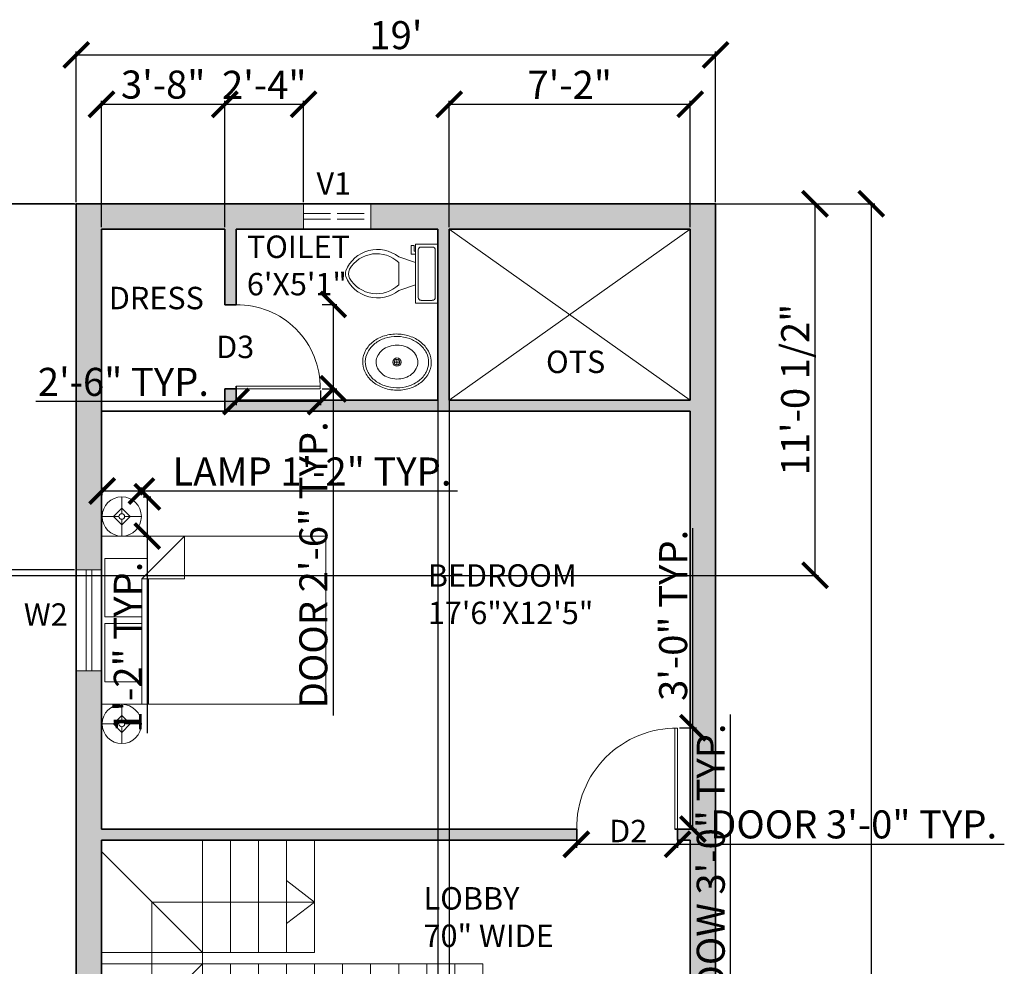
# Model space of a CAD drawing. Units: inches. Extents: x 2570 to 3313, y 1387 to 2106.
# Tile 5 of 5: x 2938 to 3289, y 1769 to 2106. Entities that reach past the tile are written whole.
import ezdxf

# ---------------------------------------------------------------- set-up
doc = ezdxf.new("R2010")
doc.units = ezdxf.units.IN
doc.linetypes.add('ACAD_ISO02W100', pattern=[15, 12, -3])
for name, color, linetype, lineweight in [('A-ANNO-DIMS', 7, 'Continuous', 18), ('A-ANNO-SYMB', 13, 'Continuous', 13), ('A-FLOR-OPEN', 8, 'Continuous', 13), ('bed', 221, 'Continuous', 18), ('DOORS', 195, 'Continuous', 18), ('P-FIXT', 8, 'Continuous', 18), ('STAIRS', 13, 'Continuous', 18), ('VENTILATORS', 143, 'ACAD_ISO02W100', 18), ('WALLS', 20, 'Continuous', 35), ('WINDOWS', 15, 'Continuous', 18)]:
    doc.layers.add(name, color=color, linetype=linetype, lineweight=lineweight)
for name, color, linetype, lineweight, true_color in [('A-ANNO-TEXT', 143, 'Continuous', 18, 0x7aafdf), ('A-AREA-IDEN', 143, 'Continuous', 18, 0x7aafdf), ('A-WALL-PATT', 30, 'Continuous', 13, 0xf26722)]:
    doc.layers.add(name, color=color, linetype=linetype, lineweight=lineweight, true_color=true_color)
doc.styles.get("Standard").update_dxf_attribs({"font": 'arial.ttf'})
doc.dimstyles.new('ISO-25', dxfattribs={"dimtxt": 10, "dimasz": 9, "dimexe": 1.25, "dimexo": 0.625, "dimtad": 1, "dimdec": 0, "dimlunit": 3, "dimtxsty": 'Standard', "dimblk": 'ARCHTICK', "dimcen": 2.5, "dimadec": 0, "dimazin": 0, "dimtfac": 1, "dimtdec": 0, "dimtmove": 0, "dimatfit": 3, "dimfxl": 1, "dimarcsym": 0})

# ---------------------------------------------------------------- blocks, each defined once
blk = doc.blocks.new('Lamp - Table')
for p, q in [((0, 7), (0, 1)), ((-1, 0), (-7, 0)), ((0, 3), (-3, 0)), ((-3, 0), (0, -3)), ((3, 0), (0, 3)), ((0, -3), (3, 0)), ((1, 0), (7, 0)), ((0, -1), (0, -7))]:
    blk.add_line(p, q)
for radius in [7, 1]:
    blk.add_circle((0, 0), radius)
blk = doc.blocks.new('Bed - Queen')
for p, q in [((0, -80.00003), (0, 0)), ((0, 0), (59.99999, 0)), ((59.99999, 0), (59.99999, -80.00003)), ((7.99999, -1.2), (28.79998, -1.2)), ((7.99999, -14.4), (7.99999, -1.2)), ((28.79998, -1.2), (28.79998, -14.4)), ((31.19999, -1.2), (51.99999, -1.2)), ((31.19999, -14.4), (31.19999, -1.2)), ((51.99999, -1.2), (51.99999, -16.4)), ((0, -14.4), (44.8, -14.4)), ((44.8, -16.8), (0, -16.8)), ((59.99999, -29.6), (44.8, -14.4)), ((44.8, -14.4), (44.8, -29.6)), ((51.99999, -16.4), (46.79936, -16.4)), ((44.8, -29.6), (59.99999, -29.6)), ((59.99999, -80.00003), (0, -80.00003))]:
    blk.add_line(p, q)
blk = doc.blocks.new('Toilet - top')
for p, q in [((9.5, -6), (9.5, -2)), ((-10, -8.5), (-8, -8.5)), ((-10, -9.5), (-10, -8.5)), ((-7, -9.5), (-10, -9.5)), ((-8, -8.5), (-8, -8)), ((-7, -8), (-7, -9.5)), ((-4, -8), (-6, -14)), ((4, -8), (6, -14)), ((4, -14), (-4, -14))]:
    blk.add_line(p, q)
blk.add_lwpolyline([(10.5, -8), (10.5, 0), (-10.5, 0), (-10.5, -8)], close=True)
for points in [[(-9.5, -2), (-9.5, -6)], [(8.5, -1), (-8.5, -1)], [(-8.5, -7), (8.5, -7)]]:
    blk.add_lwpolyline(points)
for centre, radius, start, end in [((-8.62, -1.88), 0.884, 81.8699, 188.1301), ((8.62, -1.88), 0.884, 351.8699, 98.1301), ((-8.62, -6.12), 0.884, 171.8699, 278.1301), ((8.62, -6.12), 0.884, 261.8699, 8.1301), ((3.52, -21.58), 12.17, 141.4691, 247.9714), ((4.2, -21.82), 11.33, 136.3677, 238.9468), ((-3.52, -21.58), 12.17, 292.0284, 38.5307), ((-4.2, -21.82), 11.33, 301.053, 43.6321), ((0, -27.88), 4, 245.7318, 294.2682), ((0, -29), 4, 254.8605, 285.1395)]:
    blk.add_arc(centre, radius, start, end)
blk = doc.blocks.new('Sink - Oval top')
for p, q in [((-1, 0), (1, 0)), ((0, 1), (0, -1))]:
    blk.add_line(p, q)
for points in [[(-12.23, 0.39, 0.117634), (-11.46, -3.36, 0.104469), (-8.88, -6.8, 0.090016), (-5.08, -9.07, 0.08192), (-0.32, -10.02, 0.08192), (4.49, -9.38, 0.090016), (8.42, -7.36, 0.104469), (11.22, -4.09, 0.117634), (12.23, -0.39, 0.117634), (11.46, 3.36, 0.104469), (8.88, 6.8, 0.090016), (5.08, 9.07, 0.08192), (0.32, 10.02, 0.08192), (-4.49, 9.38, 0.090016), (-8.42, 7.36, 0.104469), (-11.22, 4.09, 0.117634)], [(-11.29, 0.16, 0.118622), (-10.52, -3.25, 0.104678), (-8.07, -6.36, 0.089562), (-4.54, -8.37, 0.081185), (-0.13, -9.15, 0.081185), (4.3, -8.49, 0.089562), (7.89, -6.58, 0.104678), (10.42, -3.55, 0.118622), (11.29, -0.16, 0.118622), (10.52, 3.25, 0.104678), (8.07, 6.36, 0.089562), (4.54, 8.37, 0.081185), (0.13, 9.15, 0.081185), (-4.3, 8.49, 0.089562), (-7.89, 6.58, 0.104678), (-10.42, 3.55, 0.118622)], [(-7.42, 0.08, 0.118283), (-6.91, -2.17, 0.104607), (-5.29, -4.21, 0.089718), (-2.97, -5.53, 0.081436), (-0.07, -6.04, 0.081436), (2.84, -5.59, 0.089718), (5.2, -4.33, 0.104607), (6.86, -2.32, 0.118283), (7.42, -0.08, 0.118283), (6.91, 2.17, 0.104607), (5.29, 4.21, 0.089718), (2.97, 5.53, 0.081436), (0.07, 6.04, 0.081436), (-2.84, 5.59, 0.089718), (-5.2, 4.33, 0.104607), (-6.86, 2.32, 0.118283)]]:
    blk.add_lwpolyline(points, format="xyb", close=True)
for radius in [1.5, 1]:
    blk.add_circle((0, 0), radius)
blk = doc.blocks.new('_ArchTick')
at = {"color": 0, "linetype": 'ByBlock', "const_width": 0.15}
blk.add_lwpolyline([(-0.5, -0.5), (0.5, 0.5)], dxfattribs=at)
blk = doc.blocks.new('*D18')
at = {"layer": 'A-ANNO-DIMS', "color": 0, "lineweight": -2, "transparency": 16777216}
for p, q in [((2958.16, 2041.11), (2958.16, 2094.86)), ((2958.16, 2093.61), (3186.16, 2093.61)), ((3186.16, 2041.11), (3186.16, 2094.86))]:
    blk.add_line(p, q, dxfattribs=at)
at = {"layer": 'Defpoints', "color": 0, "transparency": 16777216}
for p in [(3186.16, 2093.61), (2958.16, 2040.49), (3186.16, 2040.49)]:
    blk.add_point(p, dxfattribs=at)
at = {"layer": 'A-ANNO-DIMS', "color": 0, "lineweight": -2, "transparency": 16777216, "xscale": 9, "yscale": 9, "zscale": 9, "rotation": 180}
blk.add_blockref('_ArchTick', (2958.16, 2093.61), dxfattribs=at)
at = {"layer": 'A-ANNO-DIMS', "color": 0, "lineweight": -2, "transparency": 16777216, "xscale": 9, "yscale": 9, "zscale": 9}
blk.add_blockref('_ArchTick', (3186.16, 2093.61), dxfattribs=at)
at = {"layer": 'A-ANNO-DIMS', "color": 0, "transparency": 16777216, "insert": (3072.16, 2099.35), "char_height": 10, "attachment_point": 5}
blk.add_mtext("19'", dxfattribs=at)
blk = doc.blocks.new('*D19')
at = {"layer": 'A-ANNO-DIMS', "color": 0, "lineweight": -2, "transparency": 16777216}
for p, q in [((3186.79, 2040.49), (3242.94, 2040.49)), ((3241.69, 2040.49), (3241.69, 1440.49)), ((3186.79, 1440.49), (3242.94, 1440.49))]:
    blk.add_line(p, q, dxfattribs=at)
at = {"layer": 'Defpoints', "color": 0, "transparency": 16777216}
for p in [(3186.16, 2040.49), (3186.16, 1440.49), (3241.69, 1440.49)]:
    blk.add_point(p, dxfattribs=at)
at = {"layer": 'A-ANNO-DIMS', "color": 0, "lineweight": -2, "transparency": 16777216, "xscale": 9, "yscale": 9, "zscale": 9}
for p, rotation in [((3241.69, 2040.49), 90), ((3241.69, 1440.49), 270)]:
    blk.add_blockref('_ArchTick', p, dxfattribs=dict(at, rotation=rotation))
at = {"layer": 'A-ANNO-DIMS', "color": 0, "transparency": 16777216, "insert": (3235.96, 1740.49), "char_height": 10, "attachment_point": 5, "rotation": 90}
blk.add_mtext("50'", dxfattribs=at)
blk = doc.blocks.new('DOOR-SWING-30IN')
for p, q in [((0, 0), (-30, 0)), ((0, -1), (-30, -1))]:
    blk.add_line(p, q)
blk.add_arc((-0.5, -0.5), 29.5, 179.029, 270.971)
blk = doc.blocks.new('DOOR-SWING-36IN')
for p, q in [((-1, 0), (-1, 36)), ((0, 0), (0, 36))]:
    blk.add_line(p, q)
blk.add_arc((-0.5, 0.5), 35.5, 89.1931, 180.8069)
blk = doc.blocks.new('WIN-36IN')
for p, q in [((-36, 0), (-36, 9)), ((0, 0), (0, 9)), ((-36, 5.5), (0, 5.5)), ((-36, 3.5), (0, 3.5))]:
    blk.add_line(p, q)
blk = doc.blocks.new('VENT-V1-24IN')
for p, q in [((0, 0), (9, 0)), ((0, -24), (9, -24))]:
    blk.add_line(p, q)
at = {"ltscale": 0.8}
for p, q in [((3.5, -24), (3.5, 0)), ((5.5, -24), (5.5, 0))]:
    blk.add_line(p, q, dxfattribs=at)
blk = doc.blocks.new('STAIR-FLIGHT-36IN-WINDER')
for p, q in [((136, 36), (0, 36)), ((36, 36), (0, 0)), ((36, 0), (36, 36)), ((46, 0), (46, 36)), ((56, 0), (56, 36)), ((66, 0), (66, 36)), ((76, 0), (76, 36)), ((86, 0), (86, 36)), ((96, 0), (96, 36)), ((106, 0), (106, 36)), ((116, 0), (116, 36)), ((126, 0), (126, 36)), ((136, 0), (136, 36))]:
    blk.add_line(p, q)
blk = doc.blocks.new('*D33')
at = {"layer": 'A-ANNO-DIMS', "color": 0, "lineweight": -2, "transparency": 16777216}
for p, q in [((2967.39, 1936.61), (2967.39, 1939.33)), ((2981.39, 1936.61), (2981.39, 1939.33)), ((2967.39, 1938.08), (2981.39, 1938.08)), ((2981.39, 1938.08), (3094.08, 1938.08))]:
    blk.add_line(p, q, dxfattribs=at)
at = {"layer": 'Defpoints', "color": 0, "transparency": 16777216}
for p in [(2967.39, 1935.98), (2981.39, 1938.08), (2981.39, 1935.98)]:
    blk.add_point(p, dxfattribs=at)
at = {"layer": 'A-ANNO-DIMS', "color": 0, "lineweight": -2, "transparency": 16777216, "xscale": 9, "yscale": 9, "zscale": 9, "rotation": 180}
blk.add_blockref('_ArchTick', (2967.39, 1938.08), dxfattribs=at)
at = {"layer": 'A-ANNO-DIMS', "color": 0, "lineweight": -2, "transparency": 16777216, "xscale": 9, "yscale": 9, "zscale": 9}
blk.add_blockref('_ArchTick', (2981.39, 1938.08), dxfattribs=at)
at = {"layer": 'A-ANNO-DIMS', "color": 0, "transparency": 16777216, "insert": (3042.23, 1943.73), "char_height": 10, "attachment_point": 5}
blk.add_mtext('LAMP 1\'-2" TYP.', dxfattribs=at)
blk = doc.blocks.new('*D34')
at = {"layer": 'A-ANNO-DIMS', "color": 0, "lineweight": -2, "transparency": 16777216}
for p, q in [((2982.02, 1935.98), (2984.74, 1935.98)), ((2983.49, 1935.98), (2983.49, 1921.98)), ((2982.02, 1921.98), (2984.74, 1921.98)), ((2983.49, 1921.98), (2983.49, 1851.72))]:
    blk.add_line(p, q, dxfattribs=at)
at = {"layer": 'Defpoints', "color": 0, "transparency": 16777216}
for p in [(2981.39, 1935.98), (2981.39, 1921.98), (2983.49, 1921.98)]:
    blk.add_point(p, dxfattribs=at)
at = {"layer": 'A-ANNO-DIMS', "color": 0, "lineweight": -2, "transparency": 16777216, "xscale": 9, "yscale": 9, "zscale": 9}
for p, rotation in [((2983.49, 1935.98), 90), ((2983.49, 1921.98), 270)]:
    blk.add_blockref('_ArchTick', p, dxfattribs=dict(at, rotation=rotation))
at = {"layer": 'A-ANNO-DIMS', "color": 0, "transparency": 16777216, "insert": (2977.84, 1882.35), "char_height": 10, "attachment_point": 5, "rotation": 90}
blk.add_mtext('1\'-2" TYP.', dxfattribs=at)
blk = doc.blocks.new('*D35')
at = {"layer": 'A-ANNO-DIMS', "color": 0, "lineweight": -2, "transparency": 16777216}
for p, q in [((3191.56, 1721.56), (3191.56, 1858.35)), ((3186.79, 1721.56), (3192.81, 1721.56)), ((3191.56, 1685.56), (3191.56, 1721.56)), ((3186.79, 1685.56), (3192.81, 1685.56))]:
    blk.add_line(p, q, dxfattribs=at)
at = {"layer": 'Defpoints', "color": 0, "transparency": 16777216}
for p in [(3186.16, 1721.56), (3191.56, 1721.56), (3186.16, 1685.56)]:
    blk.add_point(p, dxfattribs=at)
at = {"layer": 'A-ANNO-DIMS', "color": 0, "lineweight": -2, "transparency": 16777216, "xscale": 9, "yscale": 9, "zscale": 9}
for p, rotation in [((3191.56, 1721.56), 90), ((3191.56, 1685.56), 270)]:
    blk.add_blockref('_ArchTick', p, dxfattribs=dict(at, rotation=rotation))
at = {"layer": 'A-ANNO-DIMS', "color": 0, "transparency": 16777216, "insert": (3185.76, 1794.46), "char_height": 10, "attachment_point": 5, "rotation": 90}
blk.add_mtext('WINDOW 3\'-0" TYP.', dxfattribs=at)
blk = doc.blocks.new('*D39')
at = {"layer": 'A-ANNO-DIMS', "color": 0, "lineweight": -2, "transparency": 16777216}
for p, q in [((3045.92, 2004.62), (3051.07, 2004.62)), ((3049.82, 2004.62), (3049.82, 1974.49)), ((3045.92, 1974.49), (3051.07, 1974.49)), ((3049.82, 1974.49), (3049.82, 1857.99))]:
    blk.add_line(p, q, dxfattribs=at)
at = {"layer": 'Defpoints', "color": 0, "transparency": 16777216}
for p in [(3045.3, 2004.62), (3045.3, 1974.49), (3049.82, 1974.49)]:
    blk.add_point(p, dxfattribs=at)
at = {"layer": 'A-ANNO-DIMS', "color": 0, "lineweight": -2, "transparency": 16777216, "xscale": 9, "yscale": 9, "zscale": 9}
for p, rotation in [((3049.82, 2004.62), 90), ((3049.82, 1974.49), 270)]:
    blk.add_blockref('_ArchTick', p, dxfattribs=dict(at, rotation=rotation))
at = {"layer": 'A-ANNO-DIMS', "color": 0, "transparency": 16777216, "insert": (3044.02, 1911.74), "char_height": 10, "attachment_point": 5, "rotation": 90}
blk.add_mtext('DOOR 2\'-6" TYP.', dxfattribs=at)
blk = doc.blocks.new('*D40')
at = {"layer": 'A-ANNO-DIMS', "color": 0, "lineweight": -2, "transparency": 16777216}
for p, q in [((3015.16, 1973.86), (3015.16, 1968.72)), ((3045.3, 1973.86), (3045.3, 1968.72)), ((3015.16, 1969.97), (2943.79, 1969.97)), ((3045.3, 1969.97), (3015.16, 1969.97))]:
    blk.add_line(p, q, dxfattribs=at)
at = {"layer": 'Defpoints', "color": 0, "transparency": 16777216}
for p in [(3015.16, 1974.49), (3045.3, 1974.49), (3015.16, 1969.97)]:
    blk.add_point(p, dxfattribs=at)
at = {"layer": 'A-ANNO-DIMS', "color": 0, "lineweight": -2, "transparency": 16777216, "xscale": 9, "yscale": 9, "zscale": 9, "rotation": 180}
blk.add_blockref('_ArchTick', (3015.16, 1969.97), dxfattribs=at)
at = {"layer": 'A-ANNO-DIMS', "color": 0, "lineweight": -2, "transparency": 16777216, "xscale": 9, "yscale": 9, "zscale": 9}
blk.add_blockref('_ArchTick', (3045.3, 1969.97), dxfattribs=at)
at = {"layer": 'A-ANNO-DIMS', "color": 0, "transparency": 16777216, "insert": (2974.98, 1975.7), "char_height": 10, "attachment_point": 5}
blk.add_mtext('2\'-6" TYP.', dxfattribs=at)
blk = doc.blocks.new('*D41')
at = {"layer": 'A-ANNO-DIMS', "color": 0, "lineweight": -2, "transparency": 16777216}
for p, q in [((3136.53, 1816.86), (3136.53, 1810.82)), ((3172.66, 1816.86), (3172.66, 1810.82)), ((3136.53, 1812.07), (3172.66, 1812.07)), ((3172.66, 1812.07), (3289.16, 1812.07))]:
    blk.add_line(p, q, dxfattribs=at)
at = {"layer": 'Defpoints', "color": 0, "transparency": 16777216}
for p in [(3136.53, 1817.49), (3172.66, 1817.49), (3172.66, 1812.07)]:
    blk.add_point(p, dxfattribs=at)
at = {"layer": 'A-ANNO-DIMS', "color": 0, "lineweight": -2, "transparency": 16777216, "xscale": 9, "yscale": 9, "zscale": 9, "rotation": 180}
blk.add_blockref('_ArchTick', (3136.53, 1812.07), dxfattribs=at)
at = {"layer": 'A-ANNO-DIMS', "color": 0, "lineweight": -2, "transparency": 16777216, "xscale": 9, "yscale": 9, "zscale": 9}
blk.add_blockref('_ArchTick', (3172.66, 1812.07), dxfattribs=at)
at = {"layer": 'A-ANNO-DIMS', "color": 0, "transparency": 16777216, "insert": (3235.41, 1817.87), "char_height": 10, "attachment_point": 5}
blk.add_mtext('DOOR 3\'-0" TYP.', dxfattribs=at)
blk = doc.blocks.new('*D42')
at = {"layer": 'A-ANNO-DIMS', "color": 0, "lineweight": -2, "transparency": 16777216}
for p, q in [((3178.08, 1853.62), (3178.08, 1924.82)), ((3173.29, 1853.62), (3179.33, 1853.62)), ((3178.08, 1817.49), (3178.08, 1853.62)), ((3173.29, 1817.49), (3179.33, 1817.49))]:
    blk.add_line(p, q, dxfattribs=at)
at = {"layer": 'Defpoints', "color": 0, "transparency": 16777216}
for p in [(3172.66, 1853.62), (3178.08, 1853.62), (3172.66, 1817.49)]:
    blk.add_point(p, dxfattribs=at)
at = {"layer": 'A-ANNO-DIMS', "color": 0, "lineweight": -2, "transparency": 16777216, "xscale": 9, "yscale": 9, "zscale": 9}
for p, rotation in [((3178.08, 1853.62), 90), ((3178.08, 1817.49), 270)]:
    blk.add_blockref('_ArchTick', p, dxfattribs=dict(at, rotation=rotation))
at = {"layer": 'A-ANNO-DIMS', "color": 0, "transparency": 16777216, "insert": (3172.35, 1893.72), "char_height": 10, "attachment_point": 5, "rotation": 90}
blk.add_mtext('3\'-0" TYP.', dxfattribs=at)
blk = doc.blocks.new('*D61')
at = {"layer": 'A-ANNO-DIMS', "color": 0, "lineweight": -2, "transparency": 16777216}
for p, q in [((2967.16, 2032.11), (2967.16, 2077.24)), ((2967.16, 2075.99), (3011.16, 2075.99)), ((3011.16, 2032.11), (3011.16, 2077.24))]:
    blk.add_line(p, q, dxfattribs=at)
at = {"layer": 'Defpoints', "color": 0, "transparency": 16777216}
for p in [(3011.16, 2075.99), (2967.16, 2031.49), (3011.16, 2031.49)]:
    blk.add_point(p, dxfattribs=at)
at = {"layer": 'A-ANNO-DIMS', "color": 0, "lineweight": -2, "transparency": 16777216, "xscale": 9, "yscale": 9, "zscale": 9, "rotation": 180}
blk.add_blockref('_ArchTick', (2967.16, 2075.99), dxfattribs=at)
at = {"layer": 'A-ANNO-DIMS', "color": 0, "lineweight": -2, "transparency": 16777216, "xscale": 9, "yscale": 9, "zscale": 9}
blk.add_blockref('_ArchTick', (3011.16, 2075.99), dxfattribs=at)
at = {"layer": 'A-ANNO-DIMS', "color": 0, "transparency": 16777216, "insert": (2989.16, 2081.72), "char_height": 10, "attachment_point": 5}
blk.add_mtext('3\'-8"', dxfattribs=at)
blk = doc.blocks.new('*D62')
at = {"layer": 'A-ANNO-DIMS', "color": 0, "lineweight": -2, "transparency": 16777216}
for p, q in [((3091.16, 2032.11), (3091.16, 2077.24)), ((3091.16, 2075.99), (3177.16, 2075.99)), ((3177.16, 2032.11), (3177.16, 2077.24))]:
    blk.add_line(p, q, dxfattribs=at)
at = {"layer": 'Defpoints', "color": 0, "transparency": 16777216}
for p in [(3177.16, 2075.99), (3091.16, 2031.49), (3177.16, 2031.49)]:
    blk.add_point(p, dxfattribs=at)
at = {"layer": 'A-ANNO-DIMS', "color": 0, "lineweight": -2, "transparency": 16777216, "xscale": 9, "yscale": 9, "zscale": 9, "rotation": 180}
blk.add_blockref('_ArchTick', (3091.16, 2075.99), dxfattribs=at)
at = {"layer": 'A-ANNO-DIMS', "color": 0, "lineweight": -2, "transparency": 16777216, "xscale": 9, "yscale": 9, "zscale": 9}
blk.add_blockref('_ArchTick', (3177.16, 2075.99), dxfattribs=at)
at = {"layer": 'A-ANNO-DIMS', "color": 0, "transparency": 16777216, "insert": (3134.16, 2081.63), "char_height": 10, "attachment_point": 5}
blk.add_mtext('7\'-2"', dxfattribs=at)
blk = doc.blocks.new('*D67')
at = {"layer": 'A-ANNO-DIMS', "color": 0, "lineweight": -2, "transparency": 16777216}
for p, q in [((2888.78, 2040.49), (3222.91, 2040.49)), ((3221.66, 1907.99), (3221.66, 2040.49)), ((2888.78, 1907.99), (3222.91, 1907.99))]:
    blk.add_line(p, q, dxfattribs=at)
at = {"layer": 'Defpoints', "color": 0, "transparency": 16777216}
for p in [(2888.15, 2040.49), (3221.66, 2040.49), (2888.15, 1907.99)]:
    blk.add_point(p, dxfattribs=at)
at = {"layer": 'A-ANNO-DIMS', "color": 0, "lineweight": -2, "transparency": 16777216, "xscale": 9, "yscale": 9, "zscale": 9}
for p, rotation in [((3221.66, 2040.49), 90), ((3221.66, 1907.99), 270)]:
    blk.add_blockref('_ArchTick', p, dxfattribs=dict(at, rotation=rotation))
at = {"layer": 'A-ANNO-DIMS', "color": 0, "transparency": 16777216, "insert": (3215.87, 1974.24), "char_height": 10, "attachment_point": 5, "rotation": 90}
blk.add_mtext('11\'-0 1/2"', dxfattribs=at)
blk = doc.blocks.new('*D70')
at = {"layer": 'A-ANNO-DIMS', "color": 0, "lineweight": -2, "transparency": 16777216}
for p, q in [((2957.54, 2040.49), (2623.4, 2040.49)), ((2624.65, 1909.99), (2624.65, 2040.49)), ((2957.54, 1909.99), (2623.4, 1909.99))]:
    blk.add_line(p, q, dxfattribs=at)
at = {"layer": 'Defpoints', "color": 0, "transparency": 16777216}
for p in [(2624.65, 2040.49), (2958.16, 2040.49), (2958.16, 1909.99)]:
    blk.add_point(p, dxfattribs=at)
at = {"layer": 'A-ANNO-DIMS', "color": 0, "lineweight": -2, "transparency": 16777216, "xscale": 9, "yscale": 9, "zscale": 9}
for p, rotation in [((2624.65, 2040.49), 90), ((2624.65, 1909.99), 270)]:
    blk.add_blockref('_ArchTick', p, dxfattribs=dict(at, rotation=rotation))
at = {"layer": 'A-ANNO-DIMS', "color": 0, "transparency": 16777216, "insert": (2618.86, 1975.24), "char_height": 10, "attachment_point": 5, "rotation": 90}
blk.add_mtext('10\'-10 1/2"', dxfattribs=at)
blk = doc.blocks.new('*D78')
at = {"layer": 'A-ANNO-DIMS', "color": 0, "lineweight": -2, "transparency": 16777216}
for p, q in [((3011.16, 2032.11), (3011.16, 2077.24)), ((3011.16, 2075.99), (3039.26, 2075.99)), ((3039.26, 2041.11), (3039.26, 2077.24))]:
    blk.add_line(p, q, dxfattribs=at)
at = {"layer": 'Defpoints', "color": 0, "transparency": 16777216}
for p in [(3039.26, 2075.99), (3039.26, 2040.49), (3011.16, 2031.49)]:
    blk.add_point(p, dxfattribs=at)
at = {"layer": 'A-ANNO-DIMS', "color": 0, "lineweight": -2, "transparency": 16777216, "xscale": 9, "yscale": 9, "zscale": 9, "rotation": 180}
blk.add_blockref('_ArchTick', (3011.16, 2075.99), dxfattribs=at)
at = {"layer": 'A-ANNO-DIMS', "color": 0, "lineweight": -2, "transparency": 16777216, "xscale": 9, "yscale": 9, "zscale": 9}
blk.add_blockref('_ArchTick', (3039.26, 2075.99), dxfattribs=at)
at = {"layer": 'A-ANNO-DIMS', "color": 0, "transparency": 16777216, "insert": (3025.21, 2081.63), "char_height": 10, "attachment_point": 5}
blk.add_mtext('2\'-4"', dxfattribs=at)
blk = doc.blocks.new('*D79')
at = {"layer": 'A-ANNO-DIMS', "color": 0, "lineweight": -2, "transparency": 16777216}
for p, q in [((3087.16, 2030.86), (3087.16, 1403.74)), ((3091.16, 2030.86), (3091.16, 1403.74)), ((3087.16, 1404.99), (3091.16, 1404.99)), ((3091.16, 1404.99), (3128, 1404.99))]:
    blk.add_line(p, q, dxfattribs=at)
at = {"layer": 'Defpoints', "color": 0, "transparency": 16777216}
for p in [(3087.16, 2031.49), (3091.16, 2031.49), (3091.16, 1404.99)]:
    blk.add_point(p, dxfattribs=at)
at = {"layer": 'A-ANNO-DIMS', "color": 0, "lineweight": -2, "transparency": 16777216, "xscale": 9, "yscale": 9, "zscale": 9, "rotation": 180}
blk.add_blockref('_ArchTick', (3087.16, 1404.99), dxfattribs=at)
at = {"layer": 'A-ANNO-DIMS', "color": 0, "lineweight": -2, "transparency": 16777216, "xscale": 9, "yscale": 9, "zscale": 9}
blk.add_blockref('_ArchTick', (3091.16, 1404.99), dxfattribs=at)
at = {"layer": 'A-ANNO-DIMS', "color": 0, "transparency": 16777216, "insert": (3114.08, 1410.72), "char_height": 10, "attachment_point": 5}
blk.add_mtext('0\'-4"', dxfattribs=at)

msp = doc.modelspace()

# ---------------------------------------------------------------- hatches: boundary and pattern name
at = {"layer": 'A-WALL-PATT'}
h = msp.add_hatch(color=256, dxfattribs=at)
h.dxf.hatch_style = 1
h.paths.add_polyline_path([(2888.15, 1871.99), (2879.15, 1871.99), (2879.15, 1817.49), (2851.15, 1817.49), (2851.15, 1813.49), (2879.15, 1813.49), (2879.15, 1657.4), (2888.15, 1657.4)])
h.paths.add_polyline_path([(2831.15, 1737.49), (2669.15, 1737.49), (2669.15, 1813.49), (2745.15, 1813.49), (2745.15, 1849.49), (2741.15, 1849.49), (2741.15, 1817.49), (2669.15, 1817.49), (2669.15, 1838.62), (2660.15, 1838.62), (2660.15, 1669.99), (2669.15, 1669.99), (2669.15, 1728.49), (2831.15, 1728.49)])
h.paths.add_polyline_path([(2669.15, 1621.99), (2660.15, 1621.99), (2660.15, 1440.49), (2802.65, 1440.49), (2802.65, 1449.49), (2669.15, 1449.49), (2669.15, 1554.49), (2700.9, 1554.49), (2700.9, 1563.49), (2669.15, 1563.49)])
h.paths.add_polyline_path([(2780.65, 1563.49), (2748.9, 1563.49), (2748.9, 1554.49), (2780.65, 1554.49)], flags=17)
h.paths.add_polyline_path([(2836.15, 1599.49), (2879.15, 1599.49), (2879.15, 1449.49), (2874.65, 1449.49), (2874.65, 1440.49), (2888.15, 1440.49), (2888.15, 1633.4), (2879.15, 1633.4), (2879.15, 1608.49), (2831.15, 1608.49), (2831.15, 1680.49), (2827.15, 1680.49), (2827.15, 1563.49), (2822.65, 1563.49), (2822.65, 1554.49), (2836.15, 1554.49)])
h.paths.add_polyline_path([(2793.15, 1962.49), (2821.15, 1962.49), (2821.15, 1971.49), (2793.15, 1971.49), (2793.15, 2031.49), (2818.15, 2031.49), (2818.15, 2040.49), (2747.15, 2040.49), (2747.15, 2031.49), (2789.15, 2031.49), (2789.15, 1887.49), (2785.15, 1887.49), (2785.15, 1879.49), (2789.15, 1879.49), (2789.15, 1817.49), (2789.15, 1813.49), (2793.15, 1813.49), (2821.15, 1813.49), (2821.15, 1817.49), (2793.15, 1817.49)])
h.paths.add_polyline_path([(2749.15, 1887.49), (2669.15, 1887.49), (2669.15, 2031.49), (2711.15, 2031.49), (2711.15, 2040.49), (2660.15, 2040.49), (2660.15, 1862.62), (2669.15, 1862.62), (2669.15, 1883.49), (2741.15, 1883.49), (2741.15, 1879.49), (2749.15, 1879.49)])
h.paths.add_polyline_path([(2888.15, 2040.49), (2854.15, 2040.49), (2854.15, 2031.49), (2879.15, 2031.49), (2879.15, 1971.49), (2877.15, 1971.49), (2877.15, 1962.49), (2879.15, 1962.49), (2879.15, 1907.99), (2888.15, 1907.99)])
h.paths.add_polyline_path([(2967.16, 2031.49), (3011.16, 2031.49), (3011.16, 2004.49), (3015.16, 2004.49), (3015.16, 2031.49), (3039.26, 2031.49), (3039.26, 2040.49), (2958.16, 2040.49), (2958.16, 1909.99), (2967.16, 1909.99), (2967.16, 1921.99), (2967.16, 1966.49)])
h.paths.add_polyline_path([(3186.16, 2040.49), (3063.26, 2040.49), (3063.26, 2031.49), (3087.16, 2031.49), (3087.16, 1970.49), (3015.16, 1970.49), (3015.16, 1974.49), (3011.16, 1974.49), (3011.16, 1966.49), (3177.16, 1966.49), (3177.16, 1817.49), (3172.66, 1817.49), (3172.66, 1813.49), (3177.16, 1813.49), (3177.16, 1721.56), (3186.16, 1721.56)])
h.paths.add_polyline_path([(3177.16, 2031.49), (3177.16, 1970.49), (3091.16, 1970.49), (3091.16, 2031.49)], flags=16)
h.paths.add_polyline_path([(2967.16, 1873.99), (2958.16, 1873.99), (2958.16, 1712.62), (2967.16, 1712.62), (2967.16, 1724.49), (3051.16, 1724.49), (3051.16, 1710.49), (3055.16, 1710.49), (3055.16, 1724.49), (3125.16, 1724.49), (3125.16, 1676.49), (3085.16, 1676.49), (3085.16, 1672.49), (3125.16, 1672.49), (3125.16, 1668.49), (3129.16, 1668.49), (3129.16, 1733.49), (2967.16, 1733.49), (2967.16, 1813.49), (3136.66, 1813.49), (3136.66, 1817.49), (2967.16, 1817.49)])
h.paths.add_polyline_path([(2967.16, 1672.49), (3055.16, 1672.49), (3055.16, 1680.49), (3051.16, 1680.49), (3051.16, 1676.49), (2967.16, 1676.49), (2967.16, 1688.62), (2958.16, 1688.62), (2958.16, 1618.49), (2967.16, 1618.49), (2967.16, 1631.69)])
h.paths.add_polyline_path([(3186.16, 1685.56), (3177.16, 1685.56), (3177.16, 1568.09), (3169.16, 1568.09), (3169.16, 1564.09), (3177.16, 1564.09), (3177.16, 1519.49), (3177.16, 1449.49), (3186.16, 1449.49)])
h.paths.add_polyline_path([(3129.16, 1564.09), (3129.16, 1632.49), (3125.16, 1632.49), (3125.16, 1528.49), (2967.16, 1528.49), (2967.16, 1582.49), (2958.16, 1582.49), (2958.16, 1449.49), (2967.16, 1449.49), (2967.16, 1519.49), (3129.16, 1519.49)])
h.paths.add_polyline_path([(3123.16, 1975.63), (3150.13, 1975.63), (3150.13, 1992.12), (3123.16, 1992.12)], flags=8)
h.paths.add_polyline_path([(3130.18, 1590.82), (3180.42, 1590.82), (3180.42, 1617.03), (3130.18, 1617.03)], flags=9)

# ---------------------------------------------------------------- linework, layer by layer
at = {"layer": 'A-ANNO-SYMB'}
for p, q in [((3043.16, 1791.49), (3033.16, 1799.19)), ((2985.16, 1791.49), (3043.16, 1791.49)), ((2985.16, 1773.49), (2985.16, 1791.49)), ((3043.16, 1791.49), (3033.16, 1783.79)), ((2985.16, 1751.49), (2985.16, 1773.49))]:
    msp.add_line(p, q, dxfattribs=at)
at = {"layer": 'A-FLOR-OPEN'}
for p, q in [((3091.16, 1970.49), (3177.16, 2031.49)), ((3177.16, 1970.49), (3091.16, 2031.49))]:
    msp.add_line(p, q, dxfattribs=at)
at = {"layer": 'STAIRS'}
for p, q in [((3003.16, 1773.49), (3003.16, 1813.49)), ((3013.16, 1773.49), (3013.16, 1813.49)), ((3023.16, 1773.49), (3023.16, 1813.49)), ((3033.16, 1773.49), (3033.16, 1813.49)), ((3043.16, 1773.49), (3043.16, 1813.49)), ((3003.16, 1773.49), (2967.16, 1809.49)), ((2967.16, 1773.49), (3043.16, 1773.49)), ((3003.16, 1769.49), (3003.16, 1773.49))]:
    msp.add_line(p, q, dxfattribs=at)
at = {"layer": 'WALLS'}
for p, q in [((2958.16, 2040.49), (2958.16, 1440.49)), ((3186.16, 2040.49), (2958.16, 2040.49)), ((3186.16, 1440.49), (3186.16, 2040.49)), ((2967.16, 2031.49), (2967.16, 1966.49)), ((3011.16, 2031.49), (2967.16, 2031.49)), ((3011.16, 2004.49), (3011.16, 2031.49)), ((3087.16, 2031.49), (3015.16, 2031.49)), ((3015.16, 2004.49), (3015.16, 2031.49)), ((3087.16, 1970.49), (3087.16, 2031.49)), ((3177.16, 2031.49), (3091.16, 2031.49)), ((3091.16, 1970.49), (3091.16, 2031.49)), ((3177.16, 1970.49), (3177.16, 2031.49)), ((3011.16, 2004.49), (3015.16, 2004.49)), ((3011.16, 1966.49), (3011.16, 1974.49)), ((3015.16, 1974.49), (3011.16, 1974.49)), ((3015.16, 1970.49), (3015.16, 1975.49)), ((3087.16, 1970.49), (3015.16, 1970.49)), ((3177.16, 1970.49), (3091.16, 1970.49)), ((3177.16, 1966.49), (2967.16, 1966.49)), ((2967.16, 1966.49), (2967.16, 1817.49)), ((3177.16, 1817.49), (3177.16, 1966.49)), ((3136.66, 1817.49), (2967.16, 1817.49)), ((3136.66, 1817.49), (3136.66, 1813.49)), ((3177.16, 1817.49), (3171.66, 1817.49)), ((3177.16, 1817.49), (3172.66, 1817.49)), ((3172.66, 1817.49), (3172.66, 1813.49)), ((2967.16, 1813.49), (2967.16, 1733.49)), ((3136.66, 1813.49), (2967.16, 1813.49)), ((3177.16, 1813.49), (3172.66, 1813.49)), ((3177.16, 1568.09), (3177.16, 1813.49))]:
    msp.add_line(p, q, dxfattribs=at)

# ---------------------------------------------------------------- block references
at = {"layer": 'bed', "xscale": -1, "rotation": 180}
msp.add_blockref('Lamp - Table', (2974.39, 1928.98), dxfattribs=at)
at = {"layer": 'bed', "rotation": 90}
msp.add_blockref('Bed - Queen', (2967.16, 1861.99), dxfattribs=at)
at = {"layer": 'bed'}
msp.add_blockref('Lamp - Table', (2974.39, 1854.99), dxfattribs=at)
at = {"layer": 'DOORS', "rotation": 180}
msp.add_blockref('DOOR-SWING-30IN', (3015.16, 1974.49), dxfattribs=at)
at = {"layer": 'DOORS'}
msp.add_blockref('DOOR-SWING-36IN', (3172.66, 1817.49), dxfattribs=at)
at = {"layer": 'P-FIXT', "rotation": 270}
msp.add_blockref('Toilet - top', (3087.16, 2015.57), dxfattribs=at)
at = {"layer": 'P-FIXT'}
msp.add_blockref('Sink - Oval top', (3072.55, 1984.04), dxfattribs=at)
at = {"layer": 'STAIRS'}
msp.add_blockref('STAIR-FLIGHT-36IN-WINDER', (2967.16, 1733.49), dxfattribs=at)
at = {"layer": 'VENTILATORS', "rotation": 270.0000000000029}
msp.add_blockref('VENT-V1-24IN', (3063.26, 2040.49), dxfattribs=at)
at = {"layer": 'WINDOWS', "rotation": 89.99999999999935}
msp.add_blockref('WIN-36IN', (2967.16, 1909.99), dxfattribs=at)

# ---------------------------------------------------------------- texts
at = {"layer": 'A-ANNO-TEXT', "char_height": 8, "attachment_point": 1}
for s, width, insert in [('V1', 13.4987, (3043.84, 2051.76)), ('D3', 13.0839, (3008.06, 1993.46)), ('W2', 13.4987, (2939.47, 1898)), ('D2', 13.0839, (3148.22, 1820.8))]:
    msp.add_mtext_dynamic_manual_height_columns(s, width=width, gutter_width=12.5, heights=[0], dxfattribs=dict(at, insert=insert))
at = {"layer": 'A-AREA-IDEN', "char_height": 8, "attachment_point": 1}
for s, insert in [('TOILET\\P6\'X5\'1"', (3019.02, 2029.18)), ('DRESS', (2969.79, 2010.89)), ('OTS', (3125.7, 1988.14)), ('BEDROOM\\P17\'6"X12\'5"', (3083.57, 1911.93)), ('LOBBY\\P70" WIDE', (3082.03, 1796.79))]:
    msp.add_mtext_dynamic_manual_height_columns(s, width=60.8198, gutter_width=12.5, heights=[0], dxfattribs=dict(at, insert=insert))

# ---------------------------------------------------------------- dimensions: what is measured, and where the dimension line sits
at = {"layer": 'A-ANNO-DIMS'}
for base, p1, p2, override, picture, middle in [((3186.16, 2093.61), (2958.16, 2040.49), (3186.16, 2040.49), {"dimclrd": 0, "dimclre": 0, "dimclrt": 0}, '*D18', (3072.16, 2099.35)), ((3011.16, 2075.99), (2967.16, 2031.49), (3011.16, 2031.49), {"dimdec": 1, "dimlfac": 1, "dimrnd": 0, "dimzin": 1, "dimdsep": 46, "dimlunit": 4, "dimfrac": 2}, '*D61', (2989.16, 2081.72)), ((3039.26, 2075.99), (3011.16, 2031.49), (3039.26, 2040.49), {"dimdec": 1, "dimlfac": 1, "dimrnd": 0, "dimzin": 1, "dimdsep": 46, "dimlunit": 4, "dimfrac": 2}, '*D78', (3025.21, 2081.63)), ((3177.16, 2075.99), (3091.16, 2031.49), (3177.16, 2031.49), {"dimdec": 1, "dimlfac": 1, "dimrnd": 0, "dimzin": 1, "dimdsep": 46, "dimlunit": 4, "dimfrac": 2}, '*D62', (3134.16, 2081.63)), ((3091.16, 1404.99), (3087.16, 2031.49), (3091.16, 2031.49), {"dimdec": 1, "dimlfac": 1, "dimrnd": 0, "dimzin": 1, "dimdsep": 46, "dimlunit": 4, "dimfrac": 2}, '*D79', (3114.08, 1410.72))]:
    dim = msp.add_linear_dim(base=base, p1=p1, p2=p2, dimstyle='ISO-25', override=override, dxfattribs=at)
    dim.commit()
    dim.dimension.update_dxf_attribs({"geometry": picture, "text_midpoint": middle})
for base, p1, p2, override, picture, middle in [((2624.65, 2040.49), (2958.16, 1909.99), (2958.16, 2040.49), {"dimdec": 1, "dimlfac": 1, "dimrnd": 0, "dimzin": 1, "dimdsep": 46, "dimlunit": 4, "dimfrac": 2}, '*D70', (2618.86, 1975.24)), ((3221.66, 2040.49), (2888.15, 1907.99), (2888.15, 2040.49), {"dimdec": 1, "dimlfac": 1, "dimrnd": 0, "dimzin": 1, "dimdsep": 46, "dimlunit": 4, "dimfrac": 2}, '*D67', (3215.87, 1974.24)), ((3241.69, 1440.49), (3186.16, 2040.49), (3186.16, 1440.49), {"dimclrd": 0, "dimclre": 0, "dimclrt": 0}, '*D19', (3235.96, 1740.49))]:
    dim = msp.add_linear_dim(base=base, p1=p1, p2=p2, angle=90, dimstyle='ISO-25', override=override, dxfattribs=at)
    dim.commit()
    dim.dimension.update_dxf_attribs({"geometry": picture, "text_midpoint": middle})
for base, p1, p2, angle, text, picture, middle in [((3049.82, 1974.49), (3045.3, 2004.62), (3045.3, 1974.49), 270, 'DOOR <> TYP.', '*D39', (3044.02, 1911.74)), ((3015.16, 1969.97), (3045.3, 1974.49), (3015.16, 1974.49), 180, '<> TYP.', '*D40', (2974.98, 1975.7)), ((2983.49, 1921.98), (2981.39, 1935.98), (2981.39, 1921.98), 270, '<> TYP.', '*D34', (2977.84, 1882.35)), ((3178.08, 1853.62), (3172.66, 1817.49), (3172.66, 1853.62), 90, '<> TYP.', '*D42', (3172.35, 1893.72)), ((3191.56, 1721.56), (3186.16, 1685.56), (3186.16, 1721.56), 90, 'WINDOW <> TYP.', '*D35', (3185.76, 1794.46))]:
    dim = msp.add_linear_dim(base=base, p1=p1, p2=p2, angle=angle, text=text, dimstyle='ISO-25', override={"dimdec": 1, "dimlfac": 1, "dimrnd": 0, "dimzin": 1, "dimdsep": 46, "dimlunit": 4, "dimfrac": 2}, dxfattribs=at)
    dim.commit()
    dim.dimension.update_dxf_attribs({"geometry": picture, "text_midpoint": middle})
for base, p1, p2, text, picture, middle in [((2981.39, 1938.08), (2967.39, 1935.98), (2981.39, 1935.98), 'LAMP <> TYP.', '*D33', (3042.23, 1943.73)), ((3172.66, 1812.07), (3136.53, 1817.49), (3172.66, 1817.49), 'DOOR <> TYP.', '*D41', (3235.41, 1817.87))]:
    dim = msp.add_linear_dim(base=base, p1=p1, p2=p2, text=text, dimstyle='ISO-25', override={"dimdec": 1, "dimlfac": 1, "dimrnd": 0, "dimzin": 1, "dimdsep": 46, "dimlunit": 4, "dimfrac": 2}, dxfattribs=at)
    dim.commit()
    dim.dimension.update_dxf_attribs({"geometry": picture, "text_midpoint": middle})

doc.saveas('drawing.dxf')
